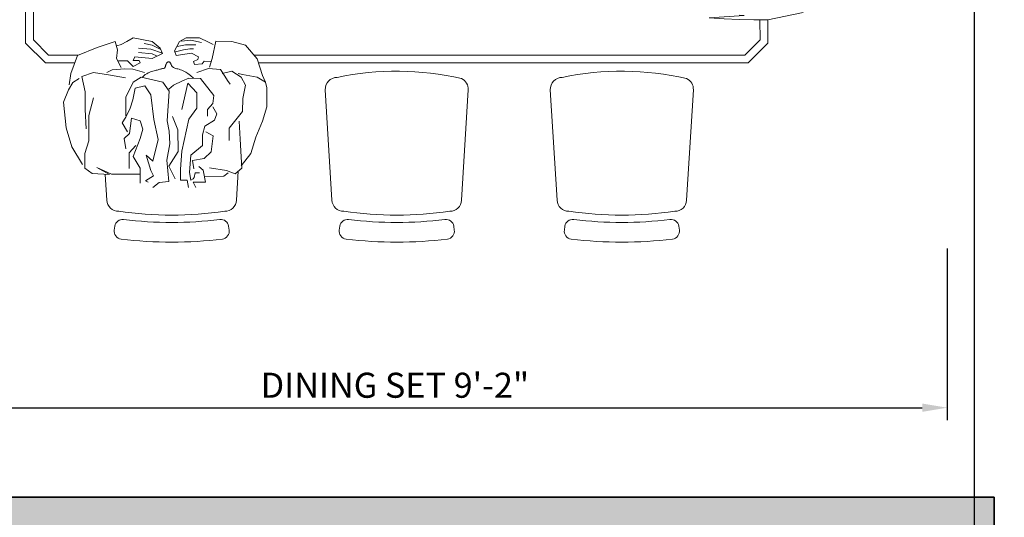
# Model space of a CAD drawing. Units: inches. Extents: x 1566 to 2546, y 1087 to 2705.
# Tile 8 of 27: x 1674 to 1773, y 1524 to 1574. Entities that reach past the tile are written whole.
import ezdxf

# ---------------------------------------------------------------- set-up
doc = ezdxf.new("R2010")
doc.units = ezdxf.units.IN
for name, color, linetype, lineweight in [('A-ANNO-DIMS', 2, 'Continuous', 18), ('A-FURN', 8, 'Continuous', 18), ('A-WALL', 7, 'Continuous', 35), ('A-WALL-PATT', 8, 'Continuous', 13)]:
    doc.layers.add(name, color=color, linetype=linetype, lineweight=lineweight)
doc.styles.get("Standard").update_dxf_attribs({"font": 'arial.ttf'})
doc.dimstyles.new('ISO-25', dxfattribs={"dimtxt": 2.5, "dimasz": 2.5, "dimexe": 1.25, "dimexo": 0.625, "dimtad": 1, "dimtxsty": 'Standard', "dimcen": 2.5, "dimadec": 0, "dimazin": 0, "dimtfac": 1, "dimtmove": 0, "dimatfit": 3, "dimfxl": 1, "dimarcsym": 0})

# ---------------------------------------------------------------- blocks, each defined once
blk = doc.blocks.new('A$C421907B3')
for p, q in [((1.2447, 2.3435), (1.2266, 2.4332)), ((1.4171, 1.0745), (1.4031, 1.0709)), ((1.4656, 1.0745), (1.4171, 1.0745)), ((1.5014, 1.0634), (1.4656, 1.0745)), ((1.3094, 1.0205), (1.3433, 1.0498)), ((1.3433, 1.0498), (1.3858, 1.0635)), ((1.3905, 1.0498), (1.3831, 1.0131)), ((1.3858, 1.0635), (1.4011, 1.0699)), ((1.4031, 1.0709), (1.3905, 1.0498)), ((1.5426, 1.0469), (1.5014, 1.0634)), ((1.5838, 1.034), (1.5426, 1.0469)), ((1.615, 1.0092), (1.5838, 1.034)), ((1.3001, 0.9856), (1.3094, 1.0205)), ((1.3751, 0.9856), (1.3904, 1.0094)), ((1.3831, 1.0131), (1.3811, 1.0021)), ((1.3904, 1.0094), (1.4104, 1.0204)), ((1.4104, 1.0204), (1.4443, 1.0139)), ((1.4443, 1.0139), (1.4768, 1.013)), ((1.4768, 1.013), (1.5193, 0.979)), ((1.5014, 1.0047), (1.5472, 1.0065)), ((1.5472, 1.0065), (1.5918, 1.0092)), ((1.5918, 1.0092), (1.621, 1.011)), ((1.621, 1.011), (1.6349, 0.9945)), ((1.2987, 0.9453), (1.3001, 0.9856)), ((1.3811, 0.9617), (1.3751, 0.9856)), ((1.3877, 0.9681), (1.3984, 0.9745)), ((1.3984, 0.9745), (1.4077, 0.9819)), ((1.5193, 0.979), (1.5505, 0.979)), ((1.6349, 0.9945), (1.627, 0.9725)), ((1.6409, 0.9652), (1.6329, 0.9762)), ((1.3678, 0.9269), (1.3705, 0.9571)), ((1.3705, 0.9571), (1.3877, 0.9681)), ((1.4655, 0.9378), (1.4827, 0.9479)), ((1.4827, 0.9479), (1.4994, 0.9423)), ((1.627, 0.9725), (1.6196, 0.9294)), ((1.6421, 0.9163), (1.6409, 0.9652)), ((1.2907, 0.904), (1.3013, 0.9269)), ((1.3432, 0.9361), (1.2987, 0.9453)), ((1.3013, 0.9269), (1.3073, 0.9388)), ((1.3645, 0.9296), (1.3432, 0.9361)), ((1.3505, 0.9315), (1.3492, 0.9159)), ((1.3784, 0.8975), (1.3678, 0.9269)), ((1.3937, 0.9067), (1.4369, 0.9406)), ((1.4369, 0.9406), (1.4568, 0.9378)), ((1.4568, 0.9378), (1.4721, 0.924)), ((1.4721, 0.924), (1.4887, 0.924)), ((1.4994, 0.9423), (1.5146, 0.9176)), ((1.5286, 0.9203), (1.5392, 0.9386)), ((1.5392, 0.9386), (1.5791, 0.9331)), ((1.5791, 0.9331), (1.5963, 0.9157)), ((1.2906, 0.87), (1.2907, 0.904)), ((1.2965, 0.8821), (1.3022, 0.9091)), ((1.3385, 0.9012), (1.3292, 0.8838)), ((1.3458, 0.8994), (1.3385, 0.9012)), ((1.3505, 0.8883), (1.3458, 0.8994)), ((1.3492, 0.9159), (1.3565, 0.9104)), ((1.3565, 0.9104), (1.3584, 0.8911)), ((1.3923, 0.8773), (1.3937, 0.9067)), ((1.5146, 0.9176), (1.5365, 0.9111)), ((1.5365, 0.9111), (1.5638, 0.9111)), ((1.5638, 0.9111), (1.5883, 0.8817)), ((1.5963, 0.9157), (1.601, 0.8863)), ((1.6163, 0.9019), (1.6256, 0.9129)), ((1.6256, 0.9129), (1.6561, 0.9193)), ((1.6329, 0.8927), (1.6329, 0.9037)), ((1.6561, 0.9193), (1.6561, 0.8881)), ((1.2985, 0.8577), (1.2965, 0.8821)), ((1.3079, 0.8681), (1.3079, 0.8945)), ((1.3183, 0.8795), (1.3183, 0.8888)), ((1.3209, 0.8634), (1.3183, 0.8795)), ((1.3292, 0.8838), (1.3351, 0.8452)), ((1.3584, 0.8911), (1.3505, 0.8883)), ((1.3774, 0.869), (1.3812, 0.8747)), ((1.3812, 0.8747), (1.3861, 0.8811)), ((1.3861, 0.8811), (1.3923, 0.8883)), ((1.3996, 0.8608), (1.3923, 0.8773)), ((1.4056, 0.8745), (1.4302, 0.8974)), ((1.472, 0.8589), (1.4056, 0.8745)), ((1.4302, 0.8974), (1.4687, 0.8974)), ((1.4687, 0.8974), (1.4966, 0.8772)), ((1.4966, 0.8772), (1.5777, 0.8588)), ((1.5883, 0.8817), (1.6315, 0.8789)), ((1.601, 0.8863), (1.6222, 0.8899)), ((1.6315, 0.8789), (1.6515, 0.8817)), ((1.6442, 0.8908), (1.6329, 0.8927)), ((1.6481, 0.8881), (1.6442, 0.8908)), ((1.6515, 0.8817), (1.6481, 0.8881)), ((1.6514, 0.8725), (1.6701, 0.8761)), ((1.6561, 0.8881), (1.6701, 0.8945)), ((1.2999, 0.8535), (1.2906, 0.87)), ((1.3232, 0.8407), (1.2999, 0.8535)), ((1.3126, 0.8473), (1.3079, 0.8681)), ((1.3261, 0.8427), (1.3209, 0.8634)), ((1.3687, 0.8462), (1.3694, 0.849)), ((1.3694, 0.849), (1.3702, 0.852)), ((1.3702, 0.852), (1.3712, 0.8555)), ((1.3712, 0.8555), (1.3726, 0.8595)), ((1.3726, 0.8595), (1.3746, 0.864)), ((1.3746, 0.864), (1.3774, 0.869)), ((1.4102, 0.8378), (1.3996, 0.8608)), ((1.49, 0.8359), (1.5239, 0.8487)), ((1.5239, 0.8487), (1.579, 0.8496)), ((1.5777, 0.8588), (1.6235, 0.856)), ((1.579, 0.8496), (1.6162, 0.8266)), ((1.6235, 0.856), (1.6514, 0.856)), ((1.6514, 0.856), (1.6514, 0.8725)), ((1.3351, 0.8452), (1.3232, 0.8407)), ((1.3512, 0.826), (1.3514, 0.8269)), ((1.3512, 0.8251), (1.3512, 0.826)), ((1.3514, 0.8243), (1.3512, 0.8251)), ((1.3514, 0.8269), (1.3518, 0.8277)), ((1.3518, 0.8234), (1.3514, 0.8243)), ((1.3518, 0.8277), (1.3524, 0.8285)), ((1.3524, 0.8226), (1.3518, 0.8234)), ((1.3524, 0.8285), (1.353, 0.8292)), ((1.353, 0.8292), (1.3538, 0.8299)), ((1.3538, 0.8299), (1.3547, 0.8305)), ((1.3547, 0.8305), (1.3557, 0.8311)), ((1.3557, 0.8311), (1.3568, 0.8316)), ((1.3568, 0.8316), (1.3579, 0.832)), ((1.3579, 0.832), (1.3591, 0.8325)), ((1.3591, 0.8325), (1.3602, 0.833)), ((1.3602, 0.833), (1.3613, 0.8335)), ((1.3613, 0.8335), (1.3624, 0.8342)), ((1.3624, 0.8342), (1.3634, 0.835)), ((1.3634, 0.835), (1.3643, 0.8359)), ((1.3643, 0.8359), (1.3651, 0.837)), ((1.3651, 0.837), (1.3659, 0.8384)), ((1.3659, 0.8384), (1.3666, 0.8399)), ((1.3666, 0.8399), (1.3673, 0.8417)), ((1.3673, 0.8417), (1.368, 0.8438)), ((1.368, 0.8438), (1.3687, 0.8462)), ((1.4029, 0.8112), (1.4255, 0.8268)), ((1.4208, 0.8259), (1.4102, 0.8378)), ((1.4255, 0.8268), (1.5012, 0.8222)), ((1.5012, 0.8222), (1.5272, 0.8267)), ((1.5272, 0.8267), (1.5591, 0.8285)), ((1.5591, 0.8285), (1.6009, 0.8212)), ((1.6009, 0.8212), (1.6547, 0.8266)), ((1.6162, 0.8266), (1.6481, 0.8422)), ((1.6547, 0.8266), (1.6574, 0.8018)), ((1.2999, 0.7838), (1.3165, 0.804)), ((1.3089, 0.784), (1.3203, 0.8058)), ((1.3165, 0.804), (1.3305, 0.8104)), ((1.3193, 0.7809), (1.3297, 0.8099)), ((1.3305, 0.8104), (1.3431, 0.7838)), ((1.3531, 0.8218), (1.3524, 0.8226)), ((1.354, 0.8211), (1.3531, 0.8218)), ((1.355, 0.8204), (1.354, 0.8211)), ((1.3561, 0.8198), (1.355, 0.8204)), ((1.3572, 0.8192), (1.3561, 0.8198)), ((1.3584, 0.8188), (1.3572, 0.8192)), ((1.3595, 0.8184), (1.3584, 0.8188)), ((1.3607, 0.8181), (1.3595, 0.8184)), ((1.3618, 0.8179), (1.3607, 0.8181)), ((1.3629, 0.8176), (1.3618, 0.8179)), ((1.3639, 0.8173), (1.3629, 0.8176)), ((1.3648, 0.8169), (1.3639, 0.8173)), ((1.3656, 0.8165), (1.3648, 0.8169)), ((1.3664, 0.8159), (1.3656, 0.8165)), ((1.367, 0.8151), (1.3664, 0.8159)), ((1.3675, 0.8141), (1.367, 0.8151)), ((1.3679, 0.813), (1.3675, 0.8141)), ((1.3683, 0.8118), (1.3679, 0.813)), ((1.3686, 0.8104), (1.3683, 0.8118)), ((1.369, 0.8088), (1.3686, 0.8104)), ((1.3694, 0.8071), (1.369, 0.8088)), ((1.3698, 0.8053), (1.3694, 0.8071)), ((1.3703, 0.8033), (1.3698, 0.8053)), ((1.3708, 0.8013), (1.3703, 0.8033)), ((1.3714, 0.799), (1.3708, 0.8013)), ((1.3721, 0.7967), (1.3714, 0.799)), ((1.3902, 0.7562), (1.4029, 0.8112)), ((1.4979, 0.7882), (1.5484, 0.7992)), ((1.5484, 0.7992), (1.6035, 0.7854)), ((1.6574, 0.8018), (1.67, 0.7853)), ((1.2905, 0.7361), (1.2999, 0.7838)), ((1.3047, 0.7638), (1.3089, 0.784)), ((1.3166, 0.7498), (1.3193, 0.7809)), ((1.3275, 0.7498), (1.3307, 0.784)), ((1.3307, 0.784), (1.3359, 0.7949)), ((1.3431, 0.7838), (1.3384, 0.7397)), ((1.3728, 0.7942), (1.3721, 0.7967)), ((1.3736, 0.7916), (1.3728, 0.7942)), ((1.3743, 0.7889), (1.3736, 0.7916)), ((1.3751, 0.786), (1.3743, 0.7889)), ((1.376, 0.783), (1.3751, 0.786)), ((1.3769, 0.7799), (1.376, 0.783)), ((1.378, 0.7767), (1.3769, 0.7799)), ((1.3795, 0.7735), (1.378, 0.7767)), ((1.3813, 0.7701), (1.3795, 0.7735)), ((1.4122, 0.7654), (1.4348, 0.7809)), ((1.4348, 0.7809), (1.4979, 0.7882)), ((1.6035, 0.7854), (1.5882, 0.7689)), ((1.5882, 0.7689), (1.6268, 0.7808)), ((1.6268, 0.7808), (1.6407, 0.7872)), ((1.6407, 0.7872), (1.6527, 0.767)), ((1.6527, 0.767), (1.656, 0.7743)), ((1.3477, 0.7507), (1.3537, 0.7535)), ((1.3477, 0.7361), (1.3477, 0.7507)), ((1.3537, 0.7535), (1.363, 0.736)), ((1.3703, 0.7351), (1.3783, 0.7645)), ((1.3837, 0.7667), (1.3813, 0.7701)), ((1.3866, 0.7633), (1.3837, 0.7667)), ((1.3902, 0.7599), (1.3866, 0.7633)), ((1.4028, 0.736), (1.3902, 0.7562)), ((1.4181, 0.7406), (1.4122, 0.7654)), ((1.4945, 0.7313), (1.5012, 0.7534)), ((1.5012, 0.7534), (1.5224, 0.7607)), ((1.5224, 0.7607), (1.5457, 0.7533)), ((1.5457, 0.7533), (1.5915, 0.7358)), ((1.5915, 0.7358), (1.6208, 0.7532)), ((1.6208, 0.7532), (1.6593, 0.7532)), ((1.6361, 0.7532), (1.636, 0.6808)), ((1.2998, 0.7196), (1.2905, 0.7361)), ((1.3384, 0.7397), (1.3477, 0.7361)), ((1.363, 0.736), (1.349, 0.7214)), ((1.3689, 0.7149), (1.3703, 0.7351)), ((1.4407, 0.7176), (1.4028, 0.736)), ((1.4473, 0.7351), (1.4181, 0.7406)), ((1.4686, 0.7286), (1.4473, 0.7351)), ((1.4918, 0.7176), (1.4686, 0.7286)), ((1.5331, 0.7267), (1.4945, 0.7313)), ((1.5457, 0.7129), (1.5331, 0.7267)), ((1.5822, 0.7258), (1.5636, 0.7423)), ((1.6221, 0.7257), (1.5822, 0.7258)), ((1.3071, 0.7058), (1.2998, 0.7196)), ((1.3104, 0.6948), (1.3071, 0.7058)), ((1.343, 0.6939), (1.3656, 0.7058)), ((1.349, 0.7214), (1.349, 0.6984)), ((1.3716, 0.6828), (1.3689, 0.7149)), ((1.3842, 0.6736), (1.3922, 0.7167)), ((1.4885, 0.7176), (1.4407, 0.7176)), ((1.5058, 0.7084), (1.4918, 0.7176)), ((1.5284, 0.7212), (1.5058, 0.7084)), ((1.5716, 0.7175), (1.5457, 0.7129)), ((1.2998, 0.6902), (1.3211, 0.6966)), ((1.315, 0.6443), (1.2998, 0.6902)), ((1.3211, 0.6966), (1.343, 0.6939)), ((1.3782, 0.6691), (1.3716, 0.6828)), ((1.3782, 0.6351), (1.3842, 0.6736)), ((1.636, 0.6808), (1.6194, 0.6441)), ((1.6194, 0.6441), (1.6373, 0.6762)), ((1.6373, 0.6762), (1.6346, 0.6321)), ((1.3349, 0.5948), (1.315, 0.6443)), ((1.3888, 0.6057), (1.3782, 0.6351)), ((1.4871, 0.624), (1.4426, 0.6351)), ((1.5516, 0.624), (1.4871, 0.624)), ((1.5835, 0.6138), (1.5516, 0.624)), ((1.6346, 0.6321), (1.6207, 0.6138)), ((1.4273, 0.614), (1.3888, 0.6057)), ((1.404, 0.5828), (1.3934, 0.5993)), ((1.4718, 0.6139), (1.4273, 0.614)), ((1.521, 0.6166), (1.4718, 0.6139)), ((1.6114, 0.6074), (1.5668, 0.5808)), ((1.6207, 0.6138), (1.5835, 0.6138)), ((1.3808, 0.5782), (1.3349, 0.5948)), ((1.41, 0.5736), (1.3808, 0.5782)), ((1.4226, 0.5718), (1.404, 0.5828)), ((1.5668, 0.5808), (1.519, 0.5662)), ((1.4532, 0.5598), (1.4226, 0.5718)), ((1.519, 0.5662), (1.4532, 0.5598))]:
    blk.add_line(p, q)
blk.add_lwpolyline([(1.2332, 2.2712), (1.2341, 2.2831), (1.2396, 2.1946), (1.2396, 2.1946), (1.2419, 2.2332), (1.2437, 2.2711), (1.2448, 2.3081), (1.2452, 2.3436)])
at = {"ltscale": 0.1}
for points in [[(1.2446, 2.3436), (1.3042, 2.3436), (1.3542, 2.2936), (1.3542, 1.0533)], [(1.245, 2.3234), (1.2959, 2.3236), (1.3342, 2.2853), (1.3342, 1.0419)], [(1.3542, 0.5878), (1.3542, 0.5135), (1.3042, 0.4635), (0.5042, 0.4635), (0.4542, 0.5135), (0.4542, 0.5377)], [(1.3342, 0.5966), (1.3342, 0.5218), (1.2959, 0.4835), (0.5125, 0.4835), (0.4742, 0.5218), (0.4742, 0.5375)]]:
    blk.add_lwpolyline(points, dxfattribs=at)
for points in [[(1.7302, 2.1079, 0.399285), (1.7017, 2.1378), (1.4223, 2.1548, 0.305593), (1.3936, 2.1375, 0.109362), (1.3908, 1.8225, 0.429301), (1.4223, 1.7925), (1.7017, 1.8094, 0.399285), (1.7302, 1.8394, 0.071734)], [(1.7584, 1.9736, -0.030867), (1.7509, 1.8517, 0.408428), (1.7679, 1.8294), (1.7778, 1.828, 0.419966), (1.8005, 1.8453, 0.030916), (1.8084, 1.9736, 0.030916), (1.8005, 2.1019, 0.419966), (1.7778, 2.1193), (1.7679, 2.1178, 0.408428), (1.7509, 2.0956, -0.030867)], [(1.7302, 1.5378, 0.399285), (1.7017, 1.5678), (1.4223, 1.5847, 0.305593), (1.3936, 1.5674, 0.109362), (1.3908, 1.2524, 0.429301), (1.4223, 1.2224), (1.7017, 1.2393, 0.399285), (1.7302, 1.2693, 0.071734)], [(1.7584, 1.4036, -0.030867), (1.7509, 1.2816, 0.408428), (1.7679, 1.2593), (1.7778, 1.2579, 0.419966), (1.8005, 1.2752, 0.030916), (1.8084, 1.4036, 0.030916), (1.8005, 1.5319, 0.419966), (1.7778, 1.5492), (1.7679, 1.5478, 0.408428), (1.7509, 1.5255, -0.030867)], [(1.7584, 0.8335, 0.030867), (1.7509, 0.9554, -0.408428), (1.7679, 0.9777), (1.7778, 0.9791, -0.419966), (1.8005, 0.9618, -0.030916), (1.8084, 0.8335, -0.030916), (1.8005, 0.7052, -0.419966), (1.7778, 0.6878), (1.7679, 0.6893, -0.408428), (1.7509, 0.7115, 0.030867)]]:
    blk.add_lwpolyline(points, format="xyb", close=True, dxfattribs=at)
blk.add_lwpolyline([(1.6285, 1.0021), (1.7017, 0.9977, -0.399285), (1.7302, 0.9677, -0.071734), (1.7302, 0.6992, -0.399285), (1.7017, 0.6693), (1.6367, 0.6653)], format="xyb", dxfattribs=at)
blk = doc.blocks.new('*D59')
at = {"layer": 'A-ANNO-DIMS', "color": 0, "lineweight": -2, "transparency": 16777216}
for p, q in [((1656.689, 1551.036), (1656.689, 1533.888)), ((1766.84, 1551.036), (1766.84, 1533.888)), ((1659.189, 1535.138), (1764.34, 1535.138))]:
    blk.add_line(p, q, dxfattribs=at)
at = {"layer": 'A-ANNO-DIMS', "color": 0, "transparency": 16777216}
for points in [[(1659.189, 1535.555), (1659.189, 1534.722), (1656.689, 1535.138)], [(1764.34, 1535.555), (1764.34, 1534.722), (1766.84, 1535.138)]]:
    blk.add_solid(points, dxfattribs=at)
at = {"layer": 'Defpoints', "color": 0, "transparency": 16777216}
for p in [(1656.689, 1551.661), (1766.84, 1551.661), (1766.84, 1535.138)]:
    blk.add_point(p, dxfattribs=at)
at = {"layer": 'A-ANNO-DIMS', "color": 0, "transparency": 16777216, "insert": (1711.764, 1537.056), "char_height": 2.5, "attachment_point": 5}
blk.add_mtext('DINING SET 9\'-2"', dxfattribs=at)
blk = doc.blocks.new('*D110')
at = {"layer": 'A-ANNO-DIMS', "color": 0, "lineweight": -2, "transparency": 16777216}
for p, q in [((1769.53, 1769.573), (1769.53, 1087.348)), ((1773.53, 1769.573), (1773.53, 1087.348)), ((1767.03, 1088.598), (1764.53, 1088.598)), ((1769.53, 1088.598), (1773.53, 1088.598)), ((1776.03, 1088.598), (1786.425, 1088.598))]:
    blk.add_line(p, q, dxfattribs=at)
at = {"layer": 'A-ANNO-DIMS', "color": 0, "transparency": 16777216}
for points in [[(1767.03, 1089.015), (1767.03, 1088.182), (1769.53, 1088.598)], [(1776.03, 1089.015), (1776.03, 1088.182), (1773.53, 1088.598)]]:
    blk.add_solid(points, dxfattribs=at)
at = {"layer": 'Defpoints', "color": 0, "transparency": 16777216}
for p in [(1769.53, 1770.198), (1773.53, 1770.198), (1773.53, 1088.598)]:
    blk.add_point(p, dxfattribs=at)
at = {"layer": 'A-ANNO-DIMS', "color": 0, "transparency": 16777216, "insert": (1782.478, 1090.5), "char_height": 2.5, "attachment_point": 5}
blk.add_mtext('0\'-4"', dxfattribs=at)

msp = doc.modelspace()

# ---------------------------------------------------------------- hatches: boundary and pattern name
at = {"layer": 'A-WALL-PATT'}
h = msp.add_hatch(color=256, dxfattribs=at)
h.dxf.hatch_style = 1
h.paths.add_polyline_path([(2001.53, 1778.198), (1641.53, 1778.198), (1641.53, 1746.198), (1649.53, 1746.198), (1649.53, 1770.198), (1769.53, 1770.198), (1769.53, 1650.198), (1767.53, 1650.198), (1767.53, 1648.198), (1767.53, 1646.198), (1819.53, 1646.198), (1819.53, 1650.198), (1773.53, 1650.198), (1773.53, 1770.198), (1941.53, 1770.198), (1941.53, 1756.195), (1945.53, 1756.195), (1945.53, 1770.198), (1993.53, 1770.198), (1993.53, 1650.198), (1945.53, 1650.198), (1945.53, 1652.198), (1943.53, 1652.198), (1941.53, 1652.198), (1941.53, 1650.198), (1867.53, 1650.198), (1867.53, 1642.198), (1871.53, 1642.198), (1871.53, 1646.198), (1993.53, 1646.198), (1993.53, 1526.198), (1871.53, 1526.198), (1871.53, 1606.198), (1867.53, 1606.198), (1867.53, 1522.198), (1993.53, 1522.198), (1993.53, 1387.198), (1959.53, 1387.198), (1959.53, 1397.198), (1955.53, 1397.198), (1955.53, 1387.198), (1903.53, 1387.198), (1903.53, 1383.198), (1993.53, 1383.198), (1993.53, 1364.301), (1993.53, 1211.198), (1939.53, 1211.198), (1939.53, 1203.198), (1993.53, 1203.198), (1993.53, 1154.198), (2001.53, 1154.198)])
h.paths.add_polyline_path([(1649.53, 1646.198), (1731.53, 1646.198), (1731.53, 1650.198), (1649.53, 1650.198), (1649.53, 1674.198), (1641.53, 1674.198), (1641.53, 1622.198), (1649.53, 1622.198)], flags=17)
h.paths.add_polyline_path([(1649.53, 1550.198), (1641.53, 1550.198), (1641.53, 1510.198), (1649.53, 1510.198), (1649.53, 1522.198), (1731.53, 1522.198), (1731.53, 1500.198), (1735.53, 1500.198), (1735.53, 1522.198), (1767.53, 1522.198), (1767.53, 1500.198), (1771.53, 1500.198), (1771.53, 1526.198), (1649.53, 1526.198)], flags=17)
h.paths.add_polyline_path([(1649.53, 1464.198), (1735.53, 1464.198), (1735.53, 1470.198), (1731.53, 1470.198), (1731.53, 1468.198), (1649.53, 1468.198), (1649.53, 1480.198), (1641.53, 1480.198), (1641.53, 1419.198), (1649.53, 1419.198)], flags=17)
h.paths.add_polyline_path([(1649.53, 1323.198), (1641.53, 1323.198), (1641.53, 1270.198), (1667.53, 1270.198), (1667.53, 1278.198), (1649.53, 1278.198)], flags=17)
h.paths.add_polyline_path([(1763.53, 1278.198), (1727.53, 1278.198), (1727.53, 1270.198), (1763.53, 1270.198)], flags=17)
h.paths.add_polyline_path([(1823.53, 1383.198), (1827.53, 1383.198), (1827.53, 1385.198), (1827.53, 1387.198), (1819.53, 1387.198), (1819.53, 1324.206), (1819.53, 1278.198), (1811.53, 1278.198), (1811.53, 1274.198), (1811.53, 1270.198), (1819.53, 1270.198), (1819.53, 1203.198), (1877.53, 1203.198), (1877.53, 1211.198), (1823.53, 1211.198)], flags=17)

# ---------------------------------------------------------------- linework, layer by layer
at = {"layer": 'A-WALL'}
for p in [(1649.53, 1526.198), (1771.53, 1500.198)]:
    msp.add_line(p, (1771.53, 1526.198), dxfattribs=at)

# ---------------------------------------------------------------- block references
at = {"layer": 'A-FURN', "xscale": 39.3701, "yscale": 39.3701, "zscale": 39.3701, "rotation": 270.0000000000005}
msp.add_blockref('A$C421907B3', (1656.689, 1622.858), dxfattribs=at)

# ---------------------------------------------------------------- dimensions: what is measured, and where the dimension line sits
at = {"layer": 'A-ANNO-DIMS'}
dim = msp.add_linear_dim(base=(1773.53, 1088.598), p1=(1769.53, 1770.198), p2=(1773.53, 1770.198), dimstyle='ISO-25', override={"dimdec": 1, "dimlfac": 1, "dimrnd": 0, "dimzin": 1, "dimdsep": 46, "dimlunit": 4, "dimfrac": 2}, dxfattribs=at)
dim.commit()
dim.dimension.update_dxf_attribs({"geometry": '*D110', "text_midpoint": (1782.478, 1090.5)})
dim = msp.add_linear_dim(base=(1766.84, 1535.138), p1=(1656.689, 1551.661), p2=(1766.84, 1551.661), angle=0, text='DINING SET <>', dimstyle='ISO-25', override={"dimdec": 1, "dimrnd": 0, "dimzin": 1, "dimlunit": 4, "dimfrac": 2}, dxfattribs=at)
dim.commit()
dim.dimension.update_dxf_attribs({"geometry": '*D59', "text_midpoint": (1711.764, 1537.056)})

doc.saveas('drawing.dxf')
